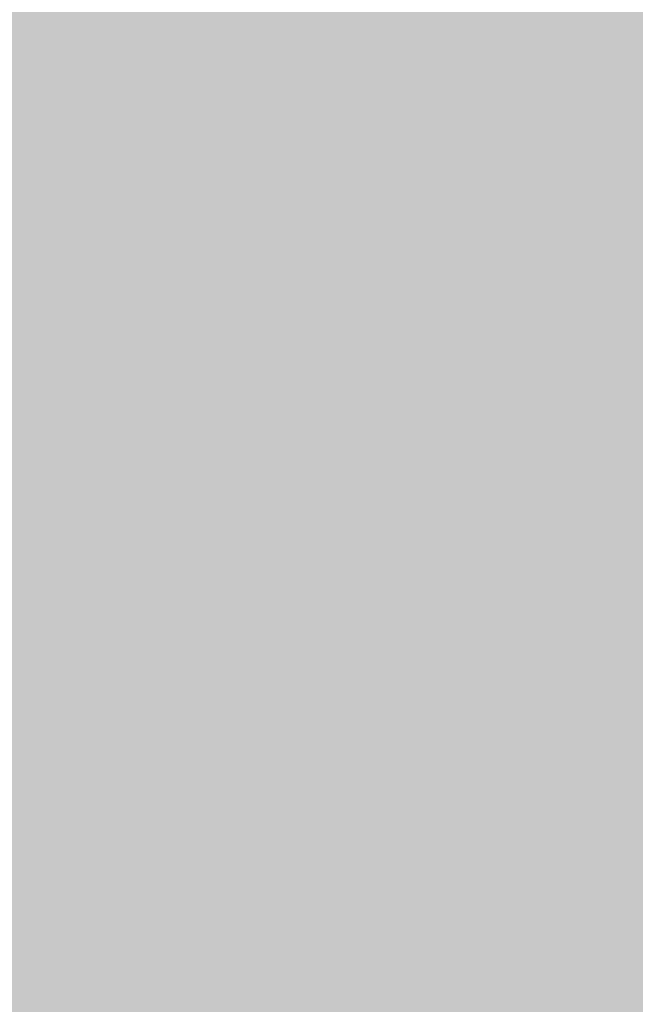
# Model space of a CAD drawing. Units: millimetres. Extents: x -22994 to 29398, y -19990 to 20176.
# Tile 84 of 135: x 229.428 to 231.767, y 79.586 to 83.328. Entities that reach past the tile are written whole.
import ezdxf
from ezdxf import colors
from ezdxf.entities.mleader import LeaderData, LeaderLine
from ezdxf.math import Vec2, Vec3

# ---------------------------------------------------------------- set-up
doc = ezdxf.new("R2010")
doc.units = ezdxf.units.MM
doc.header["$MEASUREMENT"] = 0
doc.layers.add('M-ANNO-TEXT', color=7, linetype='Continuous', lineweight=25)
doc.layers.add('M-DIMS', color=2, linetype='Continuous', lineweight=18)
doc.styles.get("Standard").update_dxf_attribs({"font": 'arial.ttf'})
doc.dimstyles.get("Standard").update_dxf_attribs({"dimtxt": 0.18, "dimasz": 10000, "dimexe": 0.18, "dimexo": 0.0625, "dimgap": 0.09, "dimtad": 0, "dimtih": 1, "dimtoh": 1, "dimdec": 0, "dimzin": 0, "dimdsep": 46, "dimtxsty": 'Standard', "dimcen": 0.09, "dimadec": 0, "dimazin": 0, "dimtfac": 1, "dimtdec": 0, "dimtofl": 0, "dimtmove": 0, "dimatfit": 3, "dimfxl": 1, "dimtolj": 1, "dimtzin": 0, "dimlwd": 30, "dimarcsym": 0})

# ---------------------------------------------------------------- blocks, each defined once
blk = doc.blocks.new('*D2')
at = {"layer": 'Defpoints', "color": 0, "transparency": 16777216}
for p in [(6.6773, 10.2713), (290.852, 10.2713), (290.852, -5.0787)]:
    blk.add_point(p, dxfattribs=at)
at = {"layer": 'M-DIMS', "color": 0, "lineweight": -2, "transparency": 16777216}
for p, q in [((6.6773, 10.2088), (6.6773, -5.2587)), ((290.852, 10.2088), (290.852, -5.2587))]:
    blk.add_line(p, q, dxfattribs=at)
at = {"layer": 'M-DIMS', "color": 0, "lineweight": 30, "transparency": 16777216}
for p, q in [((-9993.3227, -5.0787), (-19993.3227, -5.0787)), ((10290.852, -5.0787), (20290.852, -5.0787))]:
    blk.add_line(p, q, dxfattribs=at)
at = {"layer": 'M-DIMS', "color": 0, "transparency": 16777216}
for points in [[(-9993.3227, 1661.5879), (-9993.3227, -1671.7454), (6.6773, -5.0787)], [(10290.852, 1661.5879), (10290.852, -1671.7454), (290.852, -5.0787)]]:
    blk.add_solid(points, dxfattribs=at)
at = {"layer": 'M-DIMS', "color": 0, "transparency": 16777216, "insert": (148.7647, -5.0787), "char_height": 0.18, "attachment_point": 5}
blk.add_mtext('\\A1;284.2', dxfattribs=at)
blk = doc.blocks.new('*D3')
at = {"layer": 'Defpoints', "color": 0, "transparency": 16777216}
for p in [(110.2647, 204.1654), (110.2647, 176.3662), (95.8327, 127.967)]:
    blk.add_point(p, dxfattribs=at)
at = {"layer": 'M-DIMS', "color": 0, "lineweight": -2, "transparency": 16777216}
for p, q in [((95.8327, 128.0295), (95.8327, 204.3454)), ((110.2647, 176.4287), (110.2647, 204.3454))]:
    blk.add_line(p, q, dxfattribs=at)
at = {"layer": 'M-DIMS', "color": 0, "lineweight": 30, "transparency": 16777216}
for p, q in [((-9904.1673, 204.1654), (-19904.1673, 204.1654)), ((10110.2647, 204.1654), (20110.2647, 204.1654))]:
    blk.add_line(p, q, dxfattribs=at)
at = {"layer": 'M-DIMS', "color": 0, "transparency": 16777216}
for points in [[(-9904.1673, 1870.8321), (-9904.1673, -1462.5013), (95.8327, 204.1654)], [(10110.2647, 1870.8321), (10110.2647, -1462.5013), (110.2647, 204.1654)]]:
    blk.add_solid(points, dxfattribs=at)
at = {"layer": 'M-DIMS', "color": 0, "transparency": 16777216, "insert": (103.0487, 204.1654), "char_height": 0.18, "attachment_point": 5}
blk.add_mtext('\\A1;14.432', dxfattribs=at)
blk = doc.blocks.new('*D4')
at = {"layer": 'Defpoints', "color": 0, "transparency": 16777216}
for p in [(116.2647, 204.1654), (110.2647, 176.3662), (116.2647, 176.3662)]:
    blk.add_point(p, dxfattribs=at)
at = {"layer": 'M-DIMS', "color": 0, "lineweight": -2, "transparency": 16777216}
for p, q in [((110.2647, 176.4287), (110.2647, 204.3454)), ((116.2647, 176.4287), (116.2647, 204.3454))]:
    blk.add_line(p, q, dxfattribs=at)
at = {"layer": 'M-DIMS', "color": 0, "lineweight": 30, "transparency": 16777216}
for p, q in [((-9889.7353, 204.1654), (-19889.7353, 204.1654)), ((10116.2647, 204.1654), (20116.2647, 204.1654))]:
    blk.add_line(p, q, dxfattribs=at)
at = {"layer": 'M-DIMS', "color": 0, "transparency": 16777216}
for points in [[(-9889.7353, 1870.8321), (-9889.7353, -1462.5013), (110.2647, 204.1654)], [(10116.2647, 1870.8321), (10116.2647, -1462.5013), (116.2647, 204.1654)]]:
    blk.add_solid(points, dxfattribs=at)
at = {"layer": 'M-DIMS', "color": 0, "transparency": 16777216, "insert": (113.2647, 204.1654), "char_height": 0.18, "attachment_point": 5}
blk.add_mtext('\\A1;6', dxfattribs=at)
blk = doc.blocks.new('*D5')
at = {"layer": 'Defpoints', "color": 0, "transparency": 16777216}
for p in [(181.2647, 204.1654), (116.2647, 176.3662), (181.2647, 176.3662)]:
    blk.add_point(p, dxfattribs=at)
at = {"layer": 'M-DIMS', "color": 0, "lineweight": -2, "transparency": 16777216}
for p, q in [((116.2647, 176.4287), (116.2647, 204.3454)), ((181.2647, 176.4287), (181.2647, 204.3454))]:
    blk.add_line(p, q, dxfattribs=at)
at = {"layer": 'M-DIMS', "color": 0, "lineweight": 30, "transparency": 16777216}
for p, q in [((-9883.7353, 204.1654), (-19883.7353, 204.1654)), ((10181.2647, 204.1654), (20181.2647, 204.1654))]:
    blk.add_line(p, q, dxfattribs=at)
at = {"layer": 'M-DIMS', "color": 0, "transparency": 16777216}
for points in [[(-9883.7353, 1870.8321), (-9883.7353, -1462.5013), (116.2647, 204.1654)], [(10181.2647, 1870.8321), (10181.2647, -1462.5013), (181.2647, 204.1654)]]:
    blk.add_solid(points, dxfattribs=at)
at = {"layer": 'M-DIMS', "color": 0, "transparency": 16777216, "insert": (148.7647, 204.1654), "char_height": 0.18, "attachment_point": 5}
blk.add_mtext('\\A1;65', dxfattribs=at)
blk = doc.blocks.new('*D6')
at = {"layer": 'Defpoints', "color": 0, "transparency": 16777216}
for p in [(187.2647, 204.1654), (181.2647, 176.3662), (187.2647, 176.3662)]:
    blk.add_point(p, dxfattribs=at)
at = {"layer": 'M-DIMS', "color": 0, "lineweight": -2, "transparency": 16777216}
for p, q in [((181.2647, 176.4287), (181.2647, 204.3454)), ((187.2647, 176.4287), (187.2647, 204.3454))]:
    blk.add_line(p, q, dxfattribs=at)
at = {"layer": 'M-DIMS', "color": 0, "lineweight": 30, "transparency": 16777216}
for p, q in [((-9818.7353, 204.1654), (-19818.7353, 204.1654)), ((10187.2647, 204.1654), (20187.2647, 204.1654))]:
    blk.add_line(p, q, dxfattribs=at)
at = {"layer": 'M-DIMS', "color": 0, "transparency": 16777216}
for points in [[(-9818.7353, 1870.8321), (-9818.7353, -1462.5013), (181.2647, 204.1654)], [(10187.2647, 1870.8321), (10187.2647, -1462.5013), (187.2647, 204.1654)]]:
    blk.add_solid(points, dxfattribs=at)
at = {"layer": 'M-DIMS', "color": 0, "transparency": 16777216, "insert": (184.2647, 204.1654), "char_height": 0.18, "attachment_point": 5}
blk.add_mtext('\\A1;6', dxfattribs=at)
blk = doc.blocks.new('*D7')
at = {"layer": 'Defpoints', "color": 0, "transparency": 16777216}
for p in [(201.6967, 204.1654), (187.2647, 176.3662), (201.6967, 127.967)]:
    blk.add_point(p, dxfattribs=at)
at = {"layer": 'M-DIMS', "color": 0, "lineweight": -2, "transparency": 16777216}
for p, q in [((187.2647, 176.4287), (187.2647, 204.3454)), ((201.6967, 128.0295), (201.6967, 204.3454))]:
    blk.add_line(p, q, dxfattribs=at)
at = {"layer": 'M-DIMS', "color": 0, "lineweight": 30, "transparency": 16777216}
for p, q in [((-9812.7353, 204.1654), (-19812.7353, 204.1654)), ((10201.6967, 204.1654), (20201.6967, 204.1654))]:
    blk.add_line(p, q, dxfattribs=at)
at = {"layer": 'M-DIMS', "color": 0, "transparency": 16777216}
for points in [[(-9812.7353, 1870.8321), (-9812.7353, -1462.5013), (187.2647, 204.1654)], [(10201.6967, 1870.8321), (10201.6967, -1462.5013), (201.6967, 204.1654)]]:
    blk.add_solid(points, dxfattribs=at)
at = {"layer": 'M-DIMS', "color": 0, "transparency": 16777216, "insert": (194.4807, 204.1654), "char_height": 0.18, "attachment_point": 5}
blk.add_mtext('\\A1;14.432', dxfattribs=at)
blk = doc.blocks.new('*D8')
at = {"layer": 'Defpoints', "color": 0, "transparency": 16777216}
for p in [(227.6485, 204.1654), (227.6485, 146.7296), (201.6967, 127.967)]:
    blk.add_point(p, dxfattribs=at)
at = {"layer": 'M-DIMS', "color": 0, "lineweight": -2, "transparency": 16777216}
for p, q in [((201.6967, 128.0295), (201.6967, 204.3454)), ((227.6485, 146.7921), (227.6485, 204.3454))]:
    blk.add_line(p, q, dxfattribs=at)
at = {"layer": 'M-DIMS', "color": 0, "lineweight": 30, "transparency": 16777216}
for p, q in [((-9798.3033, 204.1654), (-19798.3033, 204.1654)), ((10227.6485, 204.1654), (20227.6485, 204.1654))]:
    blk.add_line(p, q, dxfattribs=at)
at = {"layer": 'M-DIMS', "color": 0, "transparency": 16777216}
for points in [[(-9798.3033, 1870.8321), (-9798.3033, -1462.5013), (201.6967, 204.1654)], [(10227.6485, 1870.8321), (10227.6485, -1462.5013), (227.6485, 204.1654)]]:
    blk.add_solid(points, dxfattribs=at)
at = {"layer": 'M-DIMS', "color": 0, "transparency": 16777216, "insert": (214.6726, 204.1654), "char_height": 0.18, "attachment_point": 5}
blk.add_mtext('\\A1;25.95', dxfattribs=at)
blk = doc.blocks.new('*D9')
at = {"layer": 'Defpoints', "color": 0, "transparency": 16777216}
for p in [(187.2647, 176.3662), (306.202, 176.3662), (290.852, 10.2713)]:
    blk.add_point(p, dxfattribs=at)
at = {"layer": 'M-DIMS', "color": 0, "lineweight": 30, "transparency": 16777216}
for p, q in [((306.202, 10176.3662), (306.202, 20176.3662)), ((306.202, -9989.7287), (306.202, -19989.7287))]:
    blk.add_line(p, q, dxfattribs=at)
at = {"layer": 'M-DIMS', "color": 0, "lineweight": -2, "transparency": 16777216}
for p, q in [((187.3272, 176.3662), (306.382, 176.3662)), ((290.9145, 10.2713), (306.382, 10.2713))]:
    blk.add_line(p, q, dxfattribs=at)
at = {"layer": 'M-DIMS', "color": 0, "transparency": 16777216}
for points in [[(-1360.4646, 10176.3662), (1972.8687, 10176.3662), (306.202, 176.3662)], [(-1360.4646, -9989.7287), (1972.8687, -9989.7287), (306.202, 10.2713)]]:
    blk.add_solid(points, dxfattribs=at)
at = {"layer": 'M-DIMS', "color": 0, "transparency": 16777216, "insert": (306.202, 93.3187), "char_height": 0.18, "attachment_point": 5}
blk.add_mtext('\\A1;166.1', dxfattribs=at)
blk = doc.blocks.new('*D10')
at = {"layer": 'Defpoints', "color": 0, "transparency": 16777216}
for p in [(125.6498, 136.0713), (133.3459, 136.0713), (133.3459, -5.0787)]:
    blk.add_point(p, dxfattribs=at)
at = {"layer": 'M-DIMS', "color": 0, "lineweight": -2, "transparency": 16777216}
for p, q in [((125.6498, 136.0088), (125.6498, -5.2587)), ((133.3459, 136.0088), (133.3459, -5.2587))]:
    blk.add_line(p, q, dxfattribs=at)
at = {"layer": 'M-DIMS', "color": 0, "lineweight": 30, "transparency": 16777216}
for p, q in [((-9874.3502, -5.0787), (-19874.3502, -5.0787)), ((10133.3459, -5.0787), (20133.3459, -5.0787))]:
    blk.add_line(p, q, dxfattribs=at)
at = {"layer": 'M-DIMS', "color": 0, "transparency": 16777216}
for points in [[(-9874.3502, 1661.5879), (-9874.3502, -1671.7454), (125.6498, -5.0787)], [(10133.3459, 1661.5879), (10133.3459, -1671.7454), (133.3459, -5.0787)]]:
    blk.add_solid(points, dxfattribs=at)
at = {"layer": 'M-DIMS', "color": 0, "transparency": 16777216, "insert": (129.4978, -5.0787), "char_height": 0.18, "attachment_point": 5}
blk.add_mtext('\\A1;7.696', dxfattribs=at)
blk = doc.blocks.new('*D11')
at = {"layer": 'Defpoints', "color": 0, "transparency": 16777216}
for p in [(133.3459, 136.0713), (135.6498, 136.0713), (135.6498, -5.0787)]:
    blk.add_point(p, dxfattribs=at)
at = {"layer": 'M-DIMS', "color": 0, "lineweight": -2, "transparency": 16777216}
for p, q in [((133.3459, 136.0088), (133.3459, -5.2587)), ((135.6498, 136.0088), (135.6498, -5.2587))]:
    blk.add_line(p, q, dxfattribs=at)
at = {"layer": 'M-DIMS', "color": 0, "lineweight": 30, "transparency": 16777216}
for p, q in [((-9866.6541, -5.0787), (-19866.6541, -5.0787)), ((10135.6498, -5.0787), (20135.6498, -5.0787))]:
    blk.add_line(p, q, dxfattribs=at)
at = {"layer": 'M-DIMS', "color": 0, "transparency": 16777216}
for points in [[(-9866.6541, 1661.5879), (-9866.6541, -1671.7454), (133.3459, -5.0787)], [(10135.6498, 1661.5879), (10135.6498, -1671.7454), (135.6498, -5.0787)]]:
    blk.add_solid(points, dxfattribs=at)
at = {"layer": 'M-DIMS', "color": 0, "transparency": 16777216, "insert": (134.4978, -5.0787), "char_height": 0.18, "attachment_point": 5}
blk.add_mtext('\\A1;2.304', dxfattribs=at)
blk = doc.blocks.new('*D12')
at = {"layer": 'Defpoints', "color": 0, "transparency": 16777216}
for p in [(135.6498, 136.0713), (145.6498, 136.0713), (145.6498, -5.0787)]:
    blk.add_point(p, dxfattribs=at)
at = {"layer": 'M-DIMS', "color": 0, "lineweight": -2, "transparency": 16777216}
for p, q in [((135.6498, 136.0088), (135.6498, -5.2587)), ((145.6498, 136.0088), (145.6498, -5.2587))]:
    blk.add_line(p, q, dxfattribs=at)
at = {"layer": 'M-DIMS', "color": 0, "lineweight": 30, "transparency": 16777216}
for p, q in [((-9864.3502, -5.0787), (-19864.3502, -5.0787)), ((10145.6498, -5.0787), (20145.6498, -5.0787))]:
    blk.add_line(p, q, dxfattribs=at)
at = {"layer": 'M-DIMS', "color": 0, "transparency": 16777216}
for points in [[(-9864.3502, 1661.5879), (-9864.3502, -1671.7454), (135.6498, -5.0787)], [(10145.6498, 1661.5879), (10145.6498, -1671.7454), (145.6498, -5.0787)]]:
    blk.add_solid(points, dxfattribs=at)
at = {"layer": 'M-DIMS', "color": 0, "transparency": 16777216, "insert": (140.6498, -5.0787), "char_height": 0.18, "attachment_point": 5}
blk.add_mtext('\\A1;10', dxfattribs=at)
blk = doc.blocks.new('*D13')
at = {"layer": 'Defpoints', "color": 0, "transparency": 16777216}
for p in [(145.6498, 136.0713), (155.6498, 136.0713), (155.6498, -5.0787)]:
    blk.add_point(p, dxfattribs=at)
at = {"layer": 'M-DIMS', "color": 0, "lineweight": -2, "transparency": 16777216}
for p, q in [((145.6498, 136.0088), (145.6498, -5.2587)), ((155.6498, 136.0088), (155.6498, -5.2587))]:
    blk.add_line(p, q, dxfattribs=at)
at = {"layer": 'M-DIMS', "color": 0, "lineweight": 30, "transparency": 16777216}
for p, q in [((-9854.3502, -5.0787), (-19854.3502, -5.0787)), ((10155.6498, -5.0787), (20155.6498, -5.0787))]:
    blk.add_line(p, q, dxfattribs=at)
at = {"layer": 'M-DIMS', "color": 0, "transparency": 16777216}
for points in [[(-9854.3502, 1661.5879), (-9854.3502, -1671.7454), (145.6498, -5.0787)], [(10155.6498, 1661.5879), (10155.6498, -1671.7454), (155.6498, -5.0787)]]:
    blk.add_solid(points, dxfattribs=at)
at = {"layer": 'M-DIMS', "color": 0, "transparency": 16777216, "insert": (150.6498, -5.0787), "char_height": 0.18, "attachment_point": 5}
blk.add_mtext('\\A1;10', dxfattribs=at)
blk = doc.blocks.new('*D14')
at = {"layer": 'Defpoints', "color": 0, "transparency": 16777216}
for p in [(155.6498, 136.0713), (165.6498, 136.0713), (165.6498, -5.0787)]:
    blk.add_point(p, dxfattribs=at)
at = {"layer": 'M-DIMS', "color": 0, "lineweight": -2, "transparency": 16777216}
for p, q in [((155.6498, 136.0088), (155.6498, -5.2587)), ((165.6498, 136.0088), (165.6498, -5.2587))]:
    blk.add_line(p, q, dxfattribs=at)
at = {"layer": 'M-DIMS', "color": 0, "lineweight": 30, "transparency": 16777216}
for p, q in [((-9844.3502, -5.0787), (-19844.3502, -5.0787)), ((10165.6498, -5.0787), (20165.6498, -5.0787))]:
    blk.add_line(p, q, dxfattribs=at)
at = {"layer": 'M-DIMS', "color": 0, "transparency": 16777216}
for points in [[(-9844.3502, 1661.5879), (-9844.3502, -1671.7454), (155.6498, -5.0787)], [(10165.6498, 1661.5879), (10165.6498, -1671.7454), (165.6498, -5.0787)]]:
    blk.add_solid(points, dxfattribs=at)
at = {"layer": 'M-DIMS', "color": 0, "transparency": 16777216, "insert": (160.6498, -5.0787), "char_height": 0.18, "attachment_point": 5}
blk.add_mtext('\\A1;10', dxfattribs=at)
blk = doc.blocks.new('*D15')
at = {"layer": 'Defpoints', "color": 0, "transparency": 16777216}
for p in [(173.3459, 154.788), (173.3459, 136.0713), (306.202, 136.0713)]:
    blk.add_point(p, dxfattribs=at)
at = {"layer": 'M-DIMS', "color": 0, "lineweight": 30, "transparency": 16777216}
for p, q in [((306.202, 10154.788), (306.202, 20154.788)), ((306.202, -9863.9287), (306.202, -19863.9287))]:
    blk.add_line(p, q, dxfattribs=at)
at = {"layer": 'M-DIMS', "color": 0, "lineweight": -2, "transparency": 16777216}
for p, q in [((173.4084, 154.788), (306.382, 154.788)), ((173.4084, 136.0713), (306.382, 136.0713))]:
    blk.add_line(p, q, dxfattribs=at)
at = {"layer": 'M-DIMS', "color": 0, "transparency": 16777216}
for points in [[(-1360.4646, 10154.788), (1972.8687, 10154.788), (306.202, 154.788)], [(-1360.4646, -9863.9287), (1972.8687, -9863.9287), (306.202, 136.0713)]]:
    blk.add_solid(points, dxfattribs=at)
at = {"layer": 'M-DIMS', "color": 0, "transparency": 16777216, "insert": (306.202, 145.4297), "char_height": 0.18, "attachment_point": 5}
blk.add_mtext('\\A1;18.717', dxfattribs=at)
blk = doc.blocks.new('*D16')
at = {"layer": 'Defpoints', "color": 0, "transparency": 16777216}
for p in [(120.1702, 204.1654), (110.4658, 48.0349), (120.1702, 48.0349)]:
    blk.add_point(p, dxfattribs=at)
at = {"layer": 'M-DIMS', "color": 0, "lineweight": -2, "transparency": 16777216}
for p, q in [((110.4658, 48.0974), (110.4658, 204.3454)), ((120.1702, 48.0974), (120.1702, 204.3454))]:
    blk.add_line(p, q, dxfattribs=at)
at = {"layer": 'M-DIMS', "color": 0, "lineweight": 30, "transparency": 16777216}
for p, q in [((-9889.5342, 204.1654), (-19889.5342, 204.1654)), ((10120.1702, 204.1654), (20120.1702, 204.1654))]:
    blk.add_line(p, q, dxfattribs=at)
at = {"layer": 'M-DIMS', "color": 0, "transparency": 16777216}
for points in [[(-9889.5342, 1870.8321), (-9889.5342, -1462.5013), (110.4658, 204.1654)], [(10120.1702, 1870.8321), (10120.1702, -1462.5013), (120.1702, 204.1654)]]:
    blk.add_solid(points, dxfattribs=at)
at = {"layer": 'M-DIMS', "color": 0, "transparency": 16777216, "insert": (115.318, 204.1654), "char_height": 0.18, "attachment_point": 5}
blk.add_mtext('\\A1;9.704', dxfattribs=at)
blk = doc.blocks.new('*D17')
at = {"layer": 'Defpoints', "color": 0, "transparency": 16777216}
for p in [(126.1702, 204.1654), (120.1702, 48.0349), (126.1702, 48.0349)]:
    blk.add_point(p, dxfattribs=at)
at = {"layer": 'M-DIMS', "color": 0, "lineweight": -2, "transparency": 16777216}
for p, q in [((120.1702, 48.0974), (120.1702, 204.3454)), ((126.1702, 48.0974), (126.1702, 204.3454))]:
    blk.add_line(p, q, dxfattribs=at)
at = {"layer": 'M-DIMS', "color": 0, "lineweight": 30, "transparency": 16777216}
for p, q in [((-9879.8298, 204.1654), (-19879.8298, 204.1654)), ((10126.1702, 204.1654), (20126.1702, 204.1654))]:
    blk.add_line(p, q, dxfattribs=at)
at = {"layer": 'M-DIMS', "color": 0, "transparency": 16777216}
for points in [[(-9879.8298, 1870.8321), (-9879.8298, -1462.5013), (120.1702, 204.1654)], [(10126.1702, 1870.8321), (10126.1702, -1462.5013), (126.1702, 204.1654)]]:
    blk.add_solid(points, dxfattribs=at)
at = {"layer": 'M-DIMS', "color": 0, "transparency": 16777216, "insert": (123.1702, 204.1654), "char_height": 0.18, "attachment_point": 5}
blk.add_mtext('\\A1;6', dxfattribs=at)
blk = doc.blocks.new('*D18')
at = {"layer": 'Defpoints', "color": 0, "transparency": 16777216}
for p in [(132.1702, 204.1654), (126.1702, 48.0349), (132.1702, 48.0349)]:
    blk.add_point(p, dxfattribs=at)
at = {"layer": 'M-DIMS', "color": 0, "lineweight": -2, "transparency": 16777216}
for p, q in [((126.1702, 48.0974), (126.1702, 204.3454)), ((132.1702, 48.0974), (132.1702, 204.3454))]:
    blk.add_line(p, q, dxfattribs=at)
at = {"layer": 'M-DIMS', "color": 0, "lineweight": 30, "transparency": 16777216}
for p, q in [((-9873.8298, 204.1654), (-19873.8298, 204.1654)), ((10132.1702, 204.1654), (20132.1702, 204.1654))]:
    blk.add_line(p, q, dxfattribs=at)
at = {"layer": 'M-DIMS', "color": 0, "transparency": 16777216}
for points in [[(-9873.8298, 1870.8321), (-9873.8298, -1462.5013), (126.1702, 204.1654)], [(10132.1702, 1870.8321), (10132.1702, -1462.5013), (132.1702, 204.1654)]]:
    blk.add_solid(points, dxfattribs=at)
at = {"layer": 'M-DIMS', "color": 0, "transparency": 16777216, "insert": (129.1702, 204.1654), "char_height": 0.18, "attachment_point": 5}
blk.add_mtext('\\A1;6', dxfattribs=at)
blk = doc.blocks.new('*D19')
at = {"layer": 'Defpoints', "color": 0, "transparency": 16777216}
for p in [(138.1702, 204.1654), (132.1702, 48.0349), (138.1702, 48.0349)]:
    blk.add_point(p, dxfattribs=at)
at = {"layer": 'M-DIMS', "color": 0, "lineweight": -2, "transparency": 16777216}
for p, q in [((132.1702, 48.0974), (132.1702, 204.3454)), ((138.1702, 48.0974), (138.1702, 204.3454))]:
    blk.add_line(p, q, dxfattribs=at)
at = {"layer": 'M-DIMS', "color": 0, "lineweight": 30, "transparency": 16777216}
for p, q in [((-9867.8298, 204.1654), (-19867.8298, 204.1654)), ((10138.1702, 204.1654), (20138.1702, 204.1654))]:
    blk.add_line(p, q, dxfattribs=at)
at = {"layer": 'M-DIMS', "color": 0, "transparency": 16777216}
for points in [[(-9867.8298, 1870.8321), (-9867.8298, -1462.5013), (132.1702, 204.1654)], [(10138.1702, 1870.8321), (10138.1702, -1462.5013), (138.1702, 204.1654)]]:
    blk.add_solid(points, dxfattribs=at)
at = {"layer": 'M-DIMS', "color": 0, "transparency": 16777216, "insert": (135.1702, 204.1654), "char_height": 0.18, "attachment_point": 5}
blk.add_mtext('\\A1;6', dxfattribs=at)
blk = doc.blocks.new('*D20')
at = {"layer": 'Defpoints', "color": 0, "transparency": 16777216}
for p in [(144.1702, 204.1654), (138.1702, 48.0349), (144.1702, 48.0349)]:
    blk.add_point(p, dxfattribs=at)
at = {"layer": 'M-DIMS', "color": 0, "lineweight": -2, "transparency": 16777216}
for p, q in [((138.1702, 48.0974), (138.1702, 204.3454)), ((144.1702, 48.0974), (144.1702, 204.3454))]:
    blk.add_line(p, q, dxfattribs=at)
at = {"layer": 'M-DIMS', "color": 0, "lineweight": 30, "transparency": 16777216}
for p, q in [((-9861.8298, 204.1654), (-19861.8298, 204.1654)), ((10144.1702, 204.1654), (20144.1702, 204.1654))]:
    blk.add_line(p, q, dxfattribs=at)
at = {"layer": 'M-DIMS', "color": 0, "transparency": 16777216}
for points in [[(-9861.8298, 1870.8321), (-9861.8298, -1462.5013), (138.1702, 204.1654)], [(10144.1702, 1870.8321), (10144.1702, -1462.5013), (144.1702, 204.1654)]]:
    blk.add_solid(points, dxfattribs=at)
at = {"layer": 'M-DIMS', "color": 0, "transparency": 16777216, "insert": (141.1702, 204.1654), "char_height": 0.18, "attachment_point": 5}
blk.add_mtext('\\A1;6', dxfattribs=at)
blk = doc.blocks.new('*D21')
at = {"layer": 'Defpoints', "color": 0, "transparency": 16777216}
for p in [(149.1157, 204.1654), (144.1702, 48.0349), (149.1157, 48.0349)]:
    blk.add_point(p, dxfattribs=at)
at = {"layer": 'M-DIMS', "color": 0, "lineweight": -2, "transparency": 16777216}
for p, q in [((144.1702, 48.0974), (144.1702, 204.3454)), ((149.1157, 48.0974), (149.1157, 204.3454))]:
    blk.add_line(p, q, dxfattribs=at)
at = {"layer": 'M-DIMS', "color": 0, "lineweight": 30, "transparency": 16777216}
for p, q in [((-9855.8298, 204.1654), (-19855.8298, 204.1654)), ((10149.1157, 204.1654), (20149.1157, 204.1654))]:
    blk.add_line(p, q, dxfattribs=at)
at = {"layer": 'M-DIMS', "color": 0, "transparency": 16777216}
for points in [[(-9855.8298, 1870.8321), (-9855.8298, -1462.5013), (144.1702, 204.1654)], [(10149.1157, 1870.8321), (10149.1157, -1462.5013), (149.1157, 204.1654)]]:
    blk.add_solid(points, dxfattribs=at)
at = {"layer": 'M-DIMS', "color": 0, "transparency": 16777216, "insert": (146.6429, 204.1654), "char_height": 0.18, "attachment_point": 5}
blk.add_mtext('\\A1;4.945', dxfattribs=at)
blk = doc.blocks.new('*D22')
at = {"layer": 'Defpoints', "color": 0, "transparency": 16777216}
for p in [(149.1157, 30.9895), (155.1157, 30.9895), (155.1157, -5.0787)]:
    blk.add_point(p, dxfattribs=at)
at = {"layer": 'M-DIMS', "color": 0, "lineweight": -2, "transparency": 16777216}
for p, q in [((149.1157, 30.927), (149.1157, -5.2587)), ((155.1157, 30.927), (155.1157, -5.2587))]:
    blk.add_line(p, q, dxfattribs=at)
at = {"layer": 'M-DIMS', "color": 0, "lineweight": 30, "transparency": 16777216}
for p, q in [((-9850.8843, -5.0787), (-19850.8843, -5.0787)), ((10155.1157, -5.0787), (20155.1157, -5.0787))]:
    blk.add_line(p, q, dxfattribs=at)
at = {"layer": 'M-DIMS', "color": 0, "transparency": 16777216}
for points in [[(-9850.8843, 1661.5879), (-9850.8843, -1671.7454), (149.1157, -5.0787)], [(10155.1157, 1661.5879), (10155.1157, -1671.7454), (155.1157, -5.0787)]]:
    blk.add_solid(points, dxfattribs=at)
at = {"layer": 'M-DIMS', "color": 0, "transparency": 16777216, "insert": (152.1157, -5.0787), "char_height": 0.18, "attachment_point": 5}
blk.add_mtext('\\A1;6', dxfattribs=at)
blk = doc.blocks.new('*D23')
at = {"layer": 'Defpoints', "color": 0, "transparency": 16777216}
for p in [(155.1157, 30.9895), (161.1157, 30.9895), (161.1157, -5.0787)]:
    blk.add_point(p, dxfattribs=at)
at = {"layer": 'M-DIMS', "color": 0, "lineweight": -2, "transparency": 16777216}
for p, q in [((155.1157, 30.927), (155.1157, -5.2587)), ((161.1157, 30.927), (161.1157, -5.2587))]:
    blk.add_line(p, q, dxfattribs=at)
at = {"layer": 'M-DIMS', "color": 0, "lineweight": 30, "transparency": 16777216}
for p, q in [((-9844.8843, -5.0787), (-19844.8843, -5.0787)), ((10161.1157, -5.0787), (20161.1157, -5.0787))]:
    blk.add_line(p, q, dxfattribs=at)
at = {"layer": 'M-DIMS', "color": 0, "transparency": 16777216}
for points in [[(-9844.8843, 1661.5879), (-9844.8843, -1671.7454), (155.1157, -5.0787)], [(10161.1157, 1661.5879), (10161.1157, -1671.7454), (161.1157, -5.0787)]]:
    blk.add_solid(points, dxfattribs=at)
at = {"layer": 'M-DIMS', "color": 0, "transparency": 16777216, "insert": (158.1157, -5.0787), "char_height": 0.18, "attachment_point": 5}
blk.add_mtext('\\A1;6', dxfattribs=at)
blk = doc.blocks.new('*D24')
at = {"layer": 'Defpoints', "color": 0, "transparency": 16777216}
for p in [(161.1157, 30.9895), (166.4387, 30.9895), (166.4387, -5.0787)]:
    blk.add_point(p, dxfattribs=at)
at = {"layer": 'M-DIMS', "color": 0, "lineweight": -2, "transparency": 16777216}
for p, q in [((161.1157, 30.927), (161.1157, -5.2587)), ((166.4387, 30.927), (166.4387, -5.2587))]:
    blk.add_line(p, q, dxfattribs=at)
at = {"layer": 'M-DIMS', "color": 0, "lineweight": 30, "transparency": 16777216}
for p, q in [((-9838.8843, -5.0787), (-19838.8843, -5.0787)), ((10166.4387, -5.0787), (20166.4387, -5.0787))]:
    blk.add_line(p, q, dxfattribs=at)
at = {"layer": 'M-DIMS', "color": 0, "transparency": 16777216}
for points in [[(-9838.8843, 1661.5879), (-9838.8843, -1671.7454), (161.1157, -5.0787)], [(10166.4387, 1661.5879), (10166.4387, -1671.7454), (166.4387, -5.0787)]]:
    blk.add_solid(points, dxfattribs=at)
at = {"layer": 'M-DIMS', "color": 0, "transparency": 16777216, "insert": (163.7772, -5.0787), "char_height": 0.18, "attachment_point": 5}
blk.add_mtext('\\A1;5.323', dxfattribs=at)
blk = doc.blocks.new('*D25')
at = {"layer": 'Defpoints', "color": 0, "transparency": 16777216}
for p in [(166.4387, 30.9895), (172.4387, 30.9895), (172.4387, -5.0787)]:
    blk.add_point(p, dxfattribs=at)
at = {"layer": 'M-DIMS', "color": 0, "lineweight": -2, "transparency": 16777216}
for p, q in [((166.4387, 30.927), (166.4387, -5.2587)), ((172.4387, 30.927), (172.4387, -5.2587))]:
    blk.add_line(p, q, dxfattribs=at)
at = {"layer": 'M-DIMS', "color": 0, "lineweight": 30, "transparency": 16777216}
for p, q in [((-9833.5613, -5.0787), (-19833.5613, -5.0787)), ((10172.4387, -5.0787), (20172.4387, -5.0787))]:
    blk.add_line(p, q, dxfattribs=at)
at = {"layer": 'M-DIMS', "color": 0, "transparency": 16777216}
for points in [[(-9833.5613, 1661.5879), (-9833.5613, -1671.7454), (166.4387, -5.0787)], [(10172.4387, 1661.5879), (10172.4387, -1671.7454), (172.4387, -5.0787)]]:
    blk.add_solid(points, dxfattribs=at)
at = {"layer": 'M-DIMS', "color": 0, "transparency": 16777216, "insert": (169.4387, -5.0787), "char_height": 0.18, "attachment_point": 5}
blk.add_mtext('\\A1;6', dxfattribs=at)
blk = doc.blocks.new('*D26')
at = {"layer": 'Defpoints', "color": 0, "transparency": 16777216}
for p in [(172.4387, 30.9895), (178.4387, 30.9895), (178.4387, -5.0787)]:
    blk.add_point(p, dxfattribs=at)
at = {"layer": 'M-DIMS', "color": 0, "lineweight": -2, "transparency": 16777216}
for p, q in [((172.4387, 30.927), (172.4387, -5.2587)), ((178.4387, 30.927), (178.4387, -5.2587))]:
    blk.add_line(p, q, dxfattribs=at)
at = {"layer": 'M-DIMS', "color": 0, "lineweight": 30, "transparency": 16777216}
for p, q in [((-9827.5613, -5.0787), (-19827.5613, -5.0787)), ((10178.4387, -5.0787), (20178.4387, -5.0787))]:
    blk.add_line(p, q, dxfattribs=at)
at = {"layer": 'M-DIMS', "color": 0, "transparency": 16777216}
for points in [[(-9827.5613, 1661.5879), (-9827.5613, -1671.7454), (172.4387, -5.0787)], [(10178.4387, 1661.5879), (10178.4387, -1671.7454), (178.4387, -5.0787)]]:
    blk.add_solid(points, dxfattribs=at)
at = {"layer": 'M-DIMS', "color": 0, "transparency": 16777216, "insert": (175.4387, -5.0787), "char_height": 0.18, "attachment_point": 5}
blk.add_mtext('\\A1;6', dxfattribs=at)
blk = doc.blocks.new('*D27')
at = {"layer": 'Defpoints', "color": 0, "transparency": 16777216}
for p in [(178.4387, 30.9895), (188.1175, 30.9895), (188.1175, -5.0787)]:
    blk.add_point(p, dxfattribs=at)
at = {"layer": 'M-DIMS', "color": 0, "lineweight": -2, "transparency": 16777216}
for p, q in [((178.4387, 30.927), (178.4387, -5.2587)), ((188.1175, 30.927), (188.1175, -5.2587))]:
    blk.add_line(p, q, dxfattribs=at)
at = {"layer": 'M-DIMS', "color": 0, "lineweight": 30, "transparency": 16777216}
for p, q in [((-9821.5613, -5.0787), (-19821.5613, -5.0787)), ((10188.1175, -5.0787), (20188.1175, -5.0787))]:
    blk.add_line(p, q, dxfattribs=at)
at = {"layer": 'M-DIMS', "color": 0, "transparency": 16777216}
for points in [[(-9821.5613, 1661.5879), (-9821.5613, -1671.7454), (178.4387, -5.0787)], [(10188.1175, 1661.5879), (10188.1175, -1671.7454), (188.1175, -5.0787)]]:
    blk.add_solid(points, dxfattribs=at)
at = {"layer": 'M-DIMS', "color": 0, "transparency": 16777216, "insert": (183.2781, -5.0787), "char_height": 0.18, "attachment_point": 5}
blk.add_mtext('\\A1;9.679', dxfattribs=at)
blk = doc.blocks.new('*D28')
at = {"layer": 'Defpoints', "color": 0, "transparency": 16777216}
for p in [(188.1175, 48.0349), (306.202, 48.0349), (188.1175, 30.9895)]:
    blk.add_point(p, dxfattribs=at)
at = {"layer": 'M-DIMS', "color": 0, "lineweight": 30, "transparency": 16777216}
for p, q in [((306.202, 10048.0349), (306.202, 20048.0349)), ((306.202, -9969.0105), (306.202, -19969.0105))]:
    blk.add_line(p, q, dxfattribs=at)
at = {"layer": 'M-DIMS', "color": 0, "lineweight": -2, "transparency": 16777216}
for p, q in [((188.18, 48.0349), (306.382, 48.0349)), ((188.18, 30.9895), (306.382, 30.9895))]:
    blk.add_line(p, q, dxfattribs=at)
at = {"layer": 'M-DIMS', "color": 0, "transparency": 16777216}
for points in [[(-1360.4646, 10048.0349), (1972.8687, 10048.0349), (306.202, 48.0349)], [(-1360.4646, -9969.0105), (1972.8687, -9969.0105), (306.202, 30.9895)]]:
    blk.add_solid(points, dxfattribs=at)
at = {"layer": 'M-DIMS', "color": 0, "transparency": 16777216, "insert": (306.202, 39.5122), "char_height": 0.18, "attachment_point": 5}
blk.add_mtext('\\A1;17.045', dxfattribs=at)
blk = doc.blocks.new('*D29')
at = {"layer": 'Defpoints', "color": 0, "transparency": 16777216}
for p in [(36.8006, 80.045), (64.0296, 80.045)]:
    blk.add_point(p, dxfattribs=at)
at = {"layer": 'M-DIMS', "color": 0, "lineweight": -2, "transparency": 16777216}
for p, q in [((50.4151, 79.955), (50.4151, 80.135)), ((50.3251, 80.045), (50.5051, 80.045))]:
    blk.add_line(p, q, dxfattribs=at)
at = {"layer": 'M-DIMS', "color": 0, "lineweight": 30, "transparency": 16777216}
blk.add_line((20064.0296, 80.0303), (10064.0296, 80.0377), dxfattribs=at)
at = {"layer": 'M-DIMS', "color": 0, "transparency": 16777216}
blk.add_solid([(10064.0309, 1746.7043), (10064.0284, -1586.629), (64.0296, 80.045)], dxfattribs=at)
at = {"layer": 'M-DIMS', "color": 0, "transparency": 16777216, "insert": (20064.5213, 80.0303), "char_height": 0.18, "attachment_point": 5}
blk.add_mtext('\\A1;∅27.23', dxfattribs=at)
blk = doc.blocks.new('*D30')
at = {"layer": 'Defpoints', "color": 0, "transparency": 16777216}
for p in [(216.3148, 146.7291), (238.9821, 146.73)]:
    blk.add_point(p, dxfattribs=at)
at = {"layer": 'M-DIMS', "color": 0, "lineweight": 30, "transparency": 16777216}
blk.add_line((20238.9821, 147.4959), (10238.9821, 147.1129), dxfattribs=at)
at = {"layer": 'M-DIMS', "color": 0, "lineweight": -2, "transparency": 16777216}
for p, q in [((227.6485, 146.6396), (227.6485, 146.8196)), ((227.5585, 146.7296), (227.7385, 146.7296))]:
    blk.add_line(p, q, dxfattribs=at)
at = {"layer": 'M-DIMS', "color": 0, "transparency": 16777216}
blk.add_solid([(10238.9183, 1813.7796), (10239.0459, -1519.5537), (238.9821, 146.73)], dxfattribs=at)
at = {"layer": 'M-DIMS', "color": 0, "transparency": 16777216, "insert": (20239.5436, 147.4959), "char_height": 0.18, "attachment_point": 5}
blk.add_mtext('\\A1;∅22.667', dxfattribs=at)
blk = doc.blocks.new('*D31')
at = {"layer": 'Defpoints', "color": 0, "transparency": 16777216}
for p in [(223.1641, 146.7291), (232.1328, 146.73)]:
    blk.add_point(p, dxfattribs=at)
at = {"layer": 'M-DIMS', "color": 0, "lineweight": 30, "transparency": 16777216}
blk.add_line((20232.1327, 148.6656), (10232.1328, 147.6978), dxfattribs=at)
at = {"layer": 'M-DIMS', "color": 0, "lineweight": -2, "transparency": 16777216}
for p, q in [((227.6485, 146.6396), (227.6485, 146.8196)), ((227.5585, 146.7296), (227.7385, 146.7296))]:
    blk.add_line(p, q, dxfattribs=at)
at = {"layer": 'M-DIMS', "color": 0, "transparency": 16777216}
blk.add_solid([(10231.9715, 1814.3645), (10232.2941, -1518.9688), (232.1328, 146.73)], dxfattribs=at)
at = {"layer": 'M-DIMS', "color": 0, "transparency": 16777216, "insert": (20232.6245, 148.6656), "char_height": 0.18, "attachment_point": 5}
blk.add_mtext('\\A1;∅8.969', dxfattribs=at)
blk = doc.blocks.new('*D33')
at = {"layer": 'Defpoints', "color": 0, "transparency": 16777216}
for p in [(229.5613, 154.3773), (232.9972, 153.3509)]:
    blk.add_point(p, dxfattribs=at)
at = {"layer": 'M-DIMS', "color": 0, "lineweight": -2, "transparency": 16777216}
for p, q in [((229.5613, 154.2873), (229.5613, 154.4673)), ((229.4713, 154.3773), (229.6513, 154.3773))]:
    blk.add_line(p, q, dxfattribs=at)
at = {"layer": 'M-DIMS', "color": 0, "lineweight": 30, "transparency": 16777216}
for p, q in [((19396.3388, -5570.8378), (9814.668, -2708.7434)), ((29396.3388, -5570.8378), (19396.3388, -5570.8378))]:
    blk.add_line(p, q, dxfattribs=at)
at = {"layer": 'M-DIMS', "color": 0, "transparency": 16777216}
blk.add_solid([(10291.6837, -1111.7983), (9337.6523, -4305.6886), (232.9972, 153.3509)], dxfattribs=at)
at = {"layer": 'M-DIMS', "color": 0, "transparency": 16777216, "insert": (29397.0125, -5570.8378), "char_height": 0.18, "attachment_point": 5}
blk.add_mtext('\\A1;6X R3.586', dxfattribs=at)
blk = doc.blocks.new('*D36')
at = {"layer": 'Defpoints', "color": 0, "transparency": 16777216}
for p in [(46.39, 31.3035), (46.3875, 26.5934)]:
    blk.add_point(p, dxfattribs=at)
at = {"layer": 'M-DIMS', "color": 0, "lineweight": 30, "transparency": 16777216}
for p, q in [((57.1499, 20031.3006), (51.77, 10031.302)), ((10057.1499, 20031.3006), (57.1499, 20031.3006))]:
    blk.add_line(p, q, dxfattribs=at)
at = {"layer": 'M-DIMS', "color": 0, "lineweight": -2, "transparency": 16777216}
for p, q in [((46.3887, 28.8585), (46.3887, 29.0385)), ((46.2987, 28.9485), (46.4787, 28.9485))]:
    blk.add_line(p, q, dxfattribs=at)
at = {"layer": 'M-DIMS', "color": 0, "transparency": 16777216}
blk.add_solid([(-1614.8965, 10032.1987), (1718.4364, 10030.4054), (46.39, 31.3035)], dxfattribs=at)
at = {"layer": 'M-DIMS', "color": 0, "transparency": 16777216, "insert": (10057.5542, 20031.3006), "char_height": 0.18, "attachment_point": 5}
blk.add_mtext('\\A1;∅4.71', dxfattribs=at)

msp = doc.modelspace()

# ---------------------------------------------------------------- dimensions: what is measured, and where the dimension line sits
at = {"layer": 'M-DIMS'}
for base, p1, p2, override, picture, middle in [((306.202, 176.3662), (290.852, 10.2713), (187.2647, 176.3662), {"dimdec": 1, "dimlfac": 1, "dimrnd": 0, "dimzin": 0, "dimdsep": 46, "dimlunit": 2}, '*D9', (306.202, 93.3187)), ((306.202, 136.0713), (173.3459, 154.788), (173.3459, 136.0713), {"dimdec": 3, "dimlfac": 1, "dimrnd": 0, "dimzin": 0, "dimdsep": 46, "dimlunit": 2}, '*D15', (306.202, 145.4297)), ((306.202, 48.0349), (188.1175, 30.9895), (188.1175, 48.0349), {"dimdec": 3, "dimlfac": 1, "dimrnd": 0, "dimzin": 0, "dimdsep": 46, "dimlunit": 2}, '*D28', (306.202, 39.5122))]:
    dim = msp.add_linear_dim(base=base, p1=p1, p2=p2, angle=90, dimstyle='Standard', override=override, dxfattribs=at)
    dim.commit()
    dim.dimension.update_dxf_attribs({"geometry": picture, "text_midpoint": middle})
for p1, p2, override, picture, middle in [((46.3875, 26.5934), (46.39, 31.3035), {"dimdec": 2, "dimlfac": 1, "dimrnd": 0, "dimzin": 0, "dimdsep": 46, "dimlunit": 2}, '*D36', (10057.5542, 20031.3006)), ((223.1641, 146.7291), (232.1328, 146.73), {"dimdec": 3, "dimlfac": 1, "dimrnd": 0, "dimzin": 0, "dimdsep": 46, "dimlunit": 2}, '*D31', (20232.1327, 148.6656)), ((216.3148, 146.7291), (238.9821, 146.73), {"dimdec": 3, "dimlfac": 1, "dimrnd": 0, "dimzin": 0, "dimdsep": 46, "dimlunit": 2}, '*D30', (20238.9821, 147.4959))]:
    dim = msp.add_diameter_dim_2p(p1=p1, p2=p2, dimstyle='Standard', override=override, dxfattribs=at)
    dim.commit()
    dim.dimension.update_dxf_attribs({"geometry": picture, "text_midpoint": middle, "dimtype": 163})
for base, p1, p2, override, picture, middle in [((110.2647, 204.1654), (95.8327, 127.967), (110.2647, 176.3662), {"dimdec": 3, "dimlfac": 1, "dimrnd": 0, "dimzin": 0, "dimdsep": 46, "dimlunit": 2}, '*D3', (103.0487, 204.1654)), ((116.2647, 204.1654), (110.2647, 176.3662), (116.2647, 176.3662), {"dimdec": 0, "dimlfac": 1, "dimrnd": 0, "dimzin": 0, "dimdsep": 46, "dimlunit": 2}, '*D4', (113.2647, 204.1654)), ((120.1702, 204.1654), (110.4658, 48.0349), (120.1702, 48.0349), {"dimdec": 3, "dimlfac": 1, "dimrnd": 0, "dimzin": 0, "dimdsep": 46, "dimlunit": 2}, '*D16', (115.318, 204.1654)), ((181.2647, 204.1654), (116.2647, 176.3662), (181.2647, 176.3662), {"dimdec": 0, "dimlfac": 1, "dimrnd": 0, "dimzin": 0, "dimdsep": 46, "dimlunit": 2}, '*D5', (148.7647, 204.1654)), ((126.1702, 204.1654), (120.1702, 48.0349), (126.1702, 48.0349), {"dimdec": 0, "dimlfac": 1, "dimrnd": 0, "dimzin": 0, "dimdsep": 46, "dimlunit": 2}, '*D17', (123.1702, 204.1654)), ((132.1702, 204.1654), (126.1702, 48.0349), (132.1702, 48.0349), {"dimdec": 0, "dimlfac": 1, "dimrnd": 0, "dimzin": 0, "dimdsep": 46, "dimlunit": 2}, '*D18', (129.1702, 204.1654)), ((138.1702, 204.1654), (132.1702, 48.0349), (138.1702, 48.0349), {"dimdec": 0, "dimlfac": 1, "dimrnd": 0, "dimzin": 0, "dimdsep": 46, "dimlunit": 2}, '*D19', (135.1702, 204.1654)), ((144.1702, 204.1654), (138.1702, 48.0349), (144.1702, 48.0349), {"dimdec": 0, "dimlfac": 1, "dimrnd": 0, "dimzin": 0, "dimdsep": 46, "dimlunit": 2}, '*D20', (141.1702, 204.1654)), ((149.11567, 204.16539), (144.17023, 48.03494), (149.11567, 48.03494), {"dimdec": 3, "dimlfac": 1, "dimrnd": 0, "dimzin": 0, "dimdsep": 46, "dimlunit": 2}, '*D21', (146.64295, 204.16539)), ((187.2647, 204.1654), (181.2647, 176.3662), (187.2647, 176.3662), {"dimdec": 0, "dimlfac": 1, "dimrnd": 0, "dimzin": 0, "dimdsep": 46, "dimlunit": 2}, '*D6', (184.2647, 204.1654)), ((201.6967, 204.1654), (187.2647, 176.3662), (201.6967, 127.967), {"dimdec": 3, "dimlfac": 1, "dimrnd": 0, "dimzin": 0, "dimdsep": 46, "dimlunit": 2}, '*D7', (194.4807, 204.1654)), ((227.6485, 204.1654), (201.6967, 127.967), (227.6485, 146.7296), {"dimdec": 2, "dimlfac": 1, "dimrnd": 0, "dimzin": 0, "dimdsep": 46, "dimlunit": 2}, '*D8', (214.6726, 204.1654)), ((290.852, -5.0787), (6.6773, 10.2713), (290.852, 10.2713), {"dimdec": 1, "dimlfac": 1, "dimrnd": 0, "dimzin": 0, "dimdsep": 46, "dimlunit": 2}, '*D2', (148.7647, -5.0787)), ((133.3459, -5.0787), (125.6498, 136.0713), (133.3459, 136.0713), {"dimdec": 3, "dimlfac": 1, "dimrnd": 0, "dimzin": 0, "dimdsep": 46, "dimlunit": 2}, '*D10', (129.4978, -5.0787)), ((135.6498, -5.0787), (133.3459, 136.0713), (135.6498, 136.0713), {"dimdec": 3, "dimlfac": 1, "dimrnd": 0, "dimzin": 0, "dimdsep": 46, "dimlunit": 2}, '*D11', (134.4978, -5.0787)), ((145.6498, -5.0787), (135.6498, 136.0713), (145.6498, 136.0713), {"dimdec": 0, "dimlfac": 1, "dimrnd": 0, "dimzin": 0, "dimdsep": 46, "dimlunit": 2}, '*D12', (140.6498, -5.0787)), ((155.6498, -5.0787), (145.6498, 136.0713), (155.6498, 136.0713), {"dimdec": 0, "dimlfac": 1, "dimrnd": 0, "dimzin": 0, "dimdsep": 46, "dimlunit": 2}, '*D13', (150.6498, -5.0787)), ((155.1157, -5.0787), (149.1157, 30.9895), (155.1157, 30.9895), {"dimdec": 0, "dimlfac": 1, "dimrnd": 0, "dimzin": 0, "dimdsep": 46, "dimlunit": 2}, '*D22', (152.1157, -5.0787)), ((161.1157, -5.0787), (155.1157, 30.9895), (161.1157, 30.9895), {"dimdec": 0, "dimlfac": 1, "dimrnd": 0, "dimzin": 0, "dimdsep": 46, "dimlunit": 2}, '*D23', (158.1157, -5.0787)), ((165.6498, -5.0787), (155.6498, 136.0713), (165.6498, 136.0713), {"dimdec": 0, "dimlfac": 1, "dimrnd": 0, "dimzin": 0, "dimdsep": 46, "dimlunit": 2}, '*D14', (160.6498, -5.0787)), ((166.4387, -5.0787), (161.1157, 30.9895), (166.4387, 30.9895), {"dimdec": 3, "dimlfac": 1, "dimrnd": 0, "dimzin": 0, "dimdsep": 46, "dimlunit": 2}, '*D24', (163.7772, -5.0787)), ((172.4387, -5.0787), (166.4387, 30.9895), (172.4387, 30.9895), {"dimdec": 0, "dimlfac": 1, "dimrnd": 0, "dimzin": 0, "dimdsep": 46, "dimlunit": 2}, '*D25', (169.4387, -5.0787)), ((178.4387, -5.0787), (172.4387, 30.9895), (178.4387, 30.9895), {"dimdec": 0, "dimlfac": 1, "dimrnd": 0, "dimzin": 0, "dimdsep": 46, "dimlunit": 2}, '*D26', (175.4387, -5.0787)), ((188.1175, -5.0787), (178.4387, 30.9895), (188.1175, 30.9895), {"dimdec": 3, "dimlfac": 1, "dimrnd": 0, "dimzin": 0, "dimdsep": 46, "dimlunit": 2}, '*D27', (183.2781, -5.0787))]:
    dim = msp.add_linear_dim(base=base, p1=p1, p2=p2, dimstyle='Standard', override=override, dxfattribs=at)
    dim.commit()
    dim.dimension.update_dxf_attribs({"geometry": picture, "text_midpoint": middle})
dim = msp.add_diameter_dim_2p(p1=(36.8006, 80.045), p2=(64.0296, 80.045), dimstyle='Standard', override={"dimdec": 2, "dimlfac": 1, "dimrnd": 0, "dimzin": 0, "dimdsep": 46, "dimlunit": 2}, dxfattribs=at)
dim.commit()
dim.dimension.update_dxf_attribs({"geometry": '*D29', "text_midpoint": (20064.0296, 80.0303)})
dim = msp.add_radius_dim(center=(229.5613, 154.3773), mpoint=(232.9972, 153.3509), text='6X <>', dimstyle='Standard', override={"dimdec": 3, "dimlfac": 1, "dimrnd": 0, "dimzin": 0, "dimdsep": 46, "dimlunit": 2}, dxfattribs=at)
dim.commit()
dim.dimension.update_dxf_attribs({"geometry": '*D33', "text_midpoint": (29397.0125, -5570.8378)})

# ---------------------------------------------------------------- leaders
at = {"layer": 'M-ANNO-TEXT'}
ml = msp.add_multileader_mtext('Standard', dxfattribs=at)
ml.set_content('combustion chamber', color=256)
ml.set_leader_properties()
ml.build(insert=Vec2(0, 0))
ml.multileader.update_dxf_attribs({"dogleg_length": 0.36, "arrow_head_size": 200})
ctx = ml.context
ctx.base_point, ctx.char_height, ctx.arrow_head_size, ctx.landing_gap_size, ctx.plane_origin = Vec3(215.7321, 57.9149), 3, 200, 0.09, Vec3(189.1175, 57.9149)
notes = []
notes.append((ctx, [(0, (1, 1, 0), (215.3721, 57.9149), (1, 0), 0.36, [(0, [(189.1175, 57.9149)], 0, [])])]))
ctx.mtext.insert, ctx.mtext.flow_direction = Vec3(215.8221, 59.4394), 5
for ctx, leaders in notes:
    for number, flags, end, landing, length, lines in leaders:
        leader = LeaderData()
        leader.index, (leader.has_last_leader_line, leader.has_dogleg_vector, leader.attachment_direction) = number, flags
        leader.last_leader_point, leader.dogleg_vector, leader.dogleg_length = Vec3(end), Vec3(landing), length
        for number, points, colour, breaks in lines:
            line = LeaderLine()
            line.index, line.vertices, line.color, line.breaks = number, Vec3.list(points), colors.encode_raw_color(colour), breaks
            leader.lines.append(line)
        ctx.leaders.append(leader)

doc.saveas('drawing.dxf')
